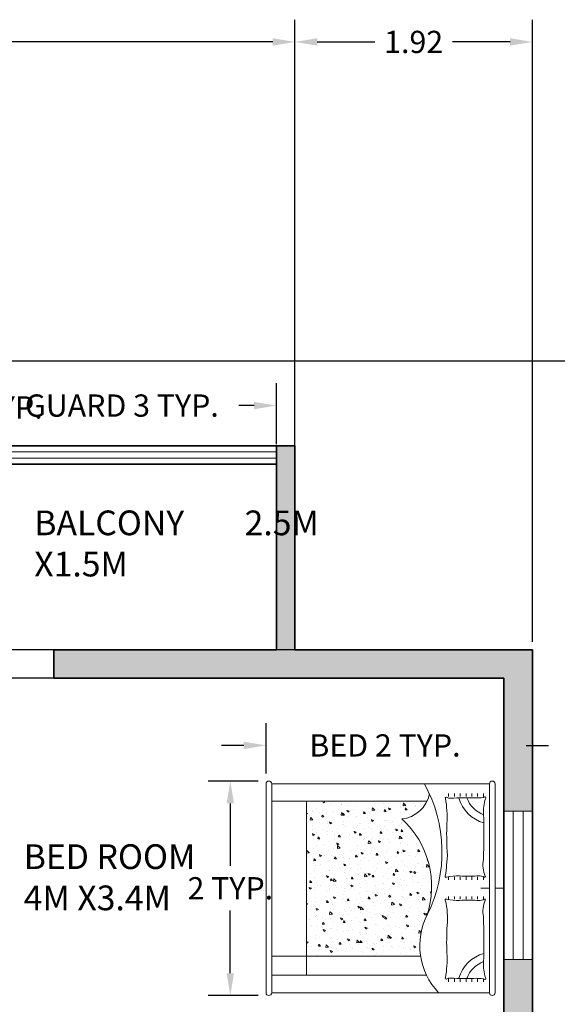
# Model space of a CAD drawing. Units: metres. Extents: x 2031 to 2061.8, y 1886.4 to 1909.8.
# Tile 10 of 10: x 2052.1 to 2056.4, y 1901.9 to 1909.8. Entities that reach past the tile are written whole.
import ezdxf

# ---------------------------------------------------------------- set-up
doc = ezdxf.new("R2010")
doc.units = ezdxf.units.M
for name, color, linetype, lineweight in [('A-ANNO-DIMS', 2, 'Continuous', 18), ('A-AREA-IDEN', 7, 'Continuous', 18), ('A-WALL-PATT', 252, 'Continuous', 13), ('furniture', 24, 'Continuous', 13), ('grills', 5, 'Continuous', 13), ('windows', 30, 'Continuous', 18)]:
    doc.layers.add(name, color=color, linetype=linetype, lineweight=lineweight)
doc.layers.add('outer walls', color=1, linetype='Continuous', lineweight=35, plot=False)
doc.styles.get("Standard").update_dxf_attribs({"font": 'arial.ttf'})
doc.dimstyles.get("Standard").update_dxf_attribs({"dimtxt": 0.18, "dimasz": 0.18, "dimexe": 0.18, "dimexo": 0.0625, "dimgap": 0.09, "dimtad": 0, "dimtih": 1, "dimtoh": 1, "dimdec": 4, "dimzin": 0, "dimdsep": 46, "dimtxsty": 'Standard', "dimcen": 0.09, "dimadec": 0, "dimazin": 0, "dimtfac": 1, "dimtdec": 4, "dimtofl": 0, "dimtmove": 0, "dimatfit": 3, "dimfxl": 1, "dimtolj": 1, "dimtzin": 0, "dimarcsym": 0})

# ---------------------------------------------------------------- blocks, each defined once
blk = doc.blocks.new('bed')
at = {"layer": 'furniture'}
h = blk.add_hatch(dxfattribs=at)
h.set_pattern_fill('AR-CONC', color=256, angle=-90.00000000000003, style=0)
h.set_pattern_definition([(320, (0, 2.380000000001032), (-0.6275213498259539, -7.172601826007534), [0.75, -8.25]), (265, (0, 2.380000000001032), (7.521921337000119, 1.387513336129997), [0.6, -6.599999999999999]), (10.45139999999999, (-0.0522933999999964, 1.782283200001032), (6.894395420609534, -5.785093817140218), [0.6374019000000001, -7.011421119999999]), (316.1842, (2, 2.380000000001032), (-1.655190143290184, -10.67241048625644), [1.125, -12.375]), (6.635599999999979, (1.862066929999997, 1.490632550001038), (9.741178709004412, -9.346627055487035), [0.956102879999999, -10.51712999999998]), (261.1842, (2, 2.380000000001032), (9.741186009253243, -9.346619451336275), [0.8999999999999989, -9.899999999999984]), (291, (1.5, 1.380000000001032), (-4.02618890665339, -5.969070521184614), [0.75, -8.25]), (236, (1.5, 1.380000000001032), (7.251500450468529, -2.433153319215819), [0.6, -6.599999999999999]), (341.4514, (1.164483939999996, 0.8825776700010266), (3.22530496709952, -8.402226285814901), [0.6374019000000001, -7.011421119999999]), (307.4999999999999, (0, 2.380000000001032), (3.328938538313114, -0.121598553172908), [0, -6.519999999999999, 0, -6.7, 0, -6.625]), (277.5, (0, 2.380000000001032), (3.944117118823601, -2.630695374421487), [0, -3.819999999999999, 0, -6.37, 0, -2.524999999999999]), (237.5, (0, 4.610000000001036), (-0.2255487173438, -5.33822436172409), [0, -2.5, 0, -7.799999999999999, 0, -10.35]), (227.5, (0, 5.610000000001036), (1.001049823323174, -5.831861693423862), [0, -3.25, 0, -5.179999999999999, 0, -7.349999999999999])])
h.paths.add_polyline_path([(30.01221964123038, -67.99999999999999), (30.01221964123036, -26.4972098666525, 0.2630430180581192), (23.90476957024844, -35.1500155485824, 0.2934236934375176), (-9.177957282599145, -26.46678060096597, -0.1566832162072435), (-23.39221964123496, -28.71851562074189), (-23.39221964123494, -67.99999999999999)])
for p, q in [((0, -3), (0, 0)), ((36.01221964123033, -3), (-36.01221964123033, -3)), ((-36.01221964123033, -5.000000000000028), (-36.01221964123027, -80)), ((36.01221964123033, -5.000000000000042), (-36.01221964123033, -5.000000000000028)), ((0, -8.000000000000043), (0, -5.000000000000042)), ((36.01221964123039, -79.99999999999999), (36.01221964123033, -5.000000000000042)), ((-31.23716250644156, -7.067621994530554), (-32.23716250644157, -7.067621994530554)), ((-31.23716250644156, -9.067621994530555), (-32.23716250644157, -9.067621994530555)), ((-3.810600647213163, -7.067621994530554), (-2.810600647213163, -7.067621994530554)), ((-3.810600647213163, -9.067621994530555), (-2.810600647213163, -9.067621994530555)), ((3.894900133777696, -7.067621994530526), (2.894900133777696, -7.067621994530526)), ((3.894900133777696, -9.067621994530526), (2.894900133777696, -9.067621994530526)), ((31.62837541028949, -7.067621994530526), (32.62837541028949, -7.067621994530526)), ((31.62837541028949, -9.067621994530526), (32.62837541028949, -9.067621994530526)), ((-31.23716250644156, -11.06762199453055), (-32.23716250644157, -11.06762199453055)), ((-31.23716250644156, -13.06762199453055), (-32.23716250644157, -13.06762199453055)), ((-3.810600647213163, -11.06762199453055), (-2.810600647213163, -11.06762199453055)), ((-3.810600647213163, -13.06762199453055), (-2.810600647213163, -13.06762199453055)), ((3.894900133777696, -11.06762199453052), (2.894900133777696, -11.06762199453052)), ((3.894900133777696, -13.06762199453052), (2.894900133777696, -13.06762199453052)), ((31.62837541028949, -11.06762199453052), (32.62837541028949, -11.06762199453052)), ((31.62837541028949, -13.06762199453052), (32.62837541028949, -13.06762199453052)), ((-31.23716250644156, -15.06762199453055), (-32.23716250644157, -15.06762199453055)), ((-3.810600647213163, -15.06762199453055), (-2.810600647213163, -15.06762199453055)), ((3.894900133777696, -15.06762199453052), (2.894900133777696, -15.06762199453052)), ((31.62837541028949, -15.06762199453052), (32.62837541028949, -15.06762199453052)), ((-31.23716250644156, -17.06762199453055), (-32.23716250644157, -17.06762199453055)), ((-31.23716250644156, -19.06762199453055), (-32.23716250644157, -19.06762199453055)), ((-3.810600647213163, -17.06762199453055), (-2.810600647213163, -17.06762199453055)), ((-3.810600647213163, -19.06762199453055), (-2.810600647213163, -19.06762199453055)), ((3.894900133777696, -17.06762199453052), (2.894900133777696, -17.06762199453052)), ((3.894900133777696, -19.06762199453052), (2.894900133777696, -19.06762199453052)), ((31.62837541028949, -17.06762199453052), (32.62837541028949, -17.06762199453052)), ((31.62837541028949, -19.06762199453052), (32.62837541028949, -19.06762199453052)), ((-36.01221964123027, -80), (36.01221964123039, -79.99999999999997)), ((-36.01221964123027, -82), (36.01221964123039, -82))]:
    blk.add_line(p, q, dxfattribs=at)
at = {"layer": 'furniture', "ltscale": 5}
blk.add_line((-30.0122196412303, -26.65900214866815), (-30.01221964123028, -80), dxfattribs=at)
at = {"layer": 'furniture', "ltscale": 7}
blk.add_line((30.01221964123039, -79.99999999999999), (30.01221964123036, -26.4972098666525), dxfattribs=at)
at = {"layer": 'furniture', "ltscale": 0.3}
for p, q in [((-23.39221964123493, -80.00000000000003), (-23.39221964123496, -28.71851562074188)), ((-30.01221964123028, -67.99999999999999), (30.01221964123039, -67.99999999999999))]:
    blk.add_line(p, q, dxfattribs=at)
at = {"layer": 'furniture'}
for centre, radius, start, end in [((-35.95310404783035, -4.000000000000014), 1.001745802777857, 93.38313670775338, 266.6168632922466), ((35.95310404783047, -4.000000000000014), 1.001745802777857, 273.3831367077534, 86.61686329224663), ((-31.09685452420217, -6.56812628935117), 0.3815901177143176, 35.89755946985184, 208.6271807330242), ((-44.4434251214767, -13.85312857714783), 14.82374463825802, 27.16285943351717, 28.62718073212637), ((-26.34909713879518, 6.677823774407073), 13.75788850886336, 251.1782289026713, 273.3982224065857), ((-8.031939823939297, 2.030581047412752), 9.294330538692307, 258.8960367609226, 294.7184225587751), ((-4.029449448298862, -6.668977911985379), 0.2818061021667602, 335.7259061638442, 114.3030308467571), ((3.223958981487498, -9.94006998173215), 7.675076275868892, 155.7259061638442, 159.0146401085631), ((4.113748934860268, -6.668977911985379), 0.2818061021635516, 65.69696915417202, 204.2740938370052), ((-3.139659494904833, -9.940069981732137), 7.675076275868892, 20.98535989143595, 24.27409383615427), ((8.116239310533615, 2.030581047735168), 9.294330539002221, 245.2815774418415, 281.1039632384965), ((26.43339662535652, 6.677823774423444), 13.75788850886336, 266.6017775934111, 288.8217710973251), ((31.18115401076358, -6.568126289351184), 0.3815901177179044, 331.3728192669758, 144.1024405301472), ((44.52772460803806, -13.85312857714784), 14.82374463825802, 151.3728192678729, 152.8371405664821), ((-46.75951437957865, -9.65138206848897), 15.71579241958107, 357.4803608088326, 9.395608387614068), ((-34.45294545533051, -3.506108501804959), 9.853247350176973, 289.8695209624031, 338.9842964810487), ((-34.45294545533051, -3.506108501804959), 12.47479548168961, 286.0319050224358, 344.1205283884622), ((-18.01528168092849, -163.5963416214672), 156.7209082093599, 87.00321809951629, 92.74968346925495), ((0.254091396095987, -8.800915214962217), 4.494229367051207, 159.014640107615, 186.2730421081171), ((-32.81622258778788, -12.43616332427339), 28.77528664700029, 354.3784002715227, 6.27304210895588), ((-0.1697919095242355, -8.800915214962217), 4.494229367051207, 353.7269578918828, 20.98535989238499), ((32.90052207435963, -12.43616332427341), 28.77528664700055, 173.7269578910441, 185.6215997284773), ((18.09958116748922, -163.5963416214399), 156.7209082093326, 87.2503165307418, 92.99678190048373), ((34.53724494190226, -3.506108501789682), 12.47479548168961, 195.8794716115377, 253.9680949775642), ((34.53724494190226, -3.506108501789682), 9.853247350176973, 201.0157035189505, 250.1304790375968), ((46.84381386614001, -9.651382068520647), 15.71579241958353, 170.6043916115409, 182.5196391911672), ((-28.61556435462791, 31.03444768063454), 42.31456350822244, 266.4835611990511, 266.6487421238194), ((54.88285648445511, -13.16191061182081), 85.98801403775587, 178.1208768196816, 183.3613129440673), ((-54.79855699787332, -13.1619106118885), 85.98801403775471, 356.6386870559327, 1.87912318031836), ((28.69986384117891, 31.03444768073385), 42.31456350831875, 273.3512578762066, 273.5164388009489), ((12.27920019974715, -16.10835590841725), 16.48064095036883, 177.0317121189266, 192.8677860199701), ((-12.19490071317551, -16.10835590841725), 16.48064095036894, 347.1322139800299, 2.968287881073314), ((-31.05019458355673, -19.91479358257859), 0.2912925215689113, 147.6219291273817, 311.93432899363), ((-33.19532486499685, -18.55460390606353), 2.248727139855352, 327.6219291288709, 339.224552802207), ((-34.12771521855714, -18.41167218428833), 3.177308659740759, 342.7808628527732, 3.755021134780372), ((-24.39731400277299, -58.0065508966982), 38.42172354635978, 93.51643880178425, 99.67664784205135), ((-24.51665474671893, -56.06449133928439), 36.47600066328987, 86.48356119821578, 93.51643880178425), ((-18.48842024981553, 70.49496359167773), 90.23180174042126, 267.5920770069633, 273.6328801943956), ((-10.30534078399284, -44.95285539311296), 25.51674577343078, 75.95197577712642, 95.54518109318596), ((-3.947726608991956, -19.99033763805275), 0.2654728058058112, 231.9004795059564, 52.89022406852256), ((4.032026095563765, -19.99033763805275), 0.2654728058058112, 127.1097759314774, 308.0995204940429), ((7.570216687580227, -34.67789736270967), 14.86666553287629, 87.39755039330738, 103.1191401867811), ((11.43897390287765, -34.80624327566366), 15.31635237680183, 84.69404282866213, 102.035481886755), ((18.57271973638731, 70.4949635916777), 90.23180174042125, 266.3671198056044, 272.4079229930367), ((24.6009542333012, -56.0644913392844), 36.47600066328987, 86.48356119821578, 93.51643880178425), ((24.48161348934542, -58.00655089669821), 38.42172354635978, 80.32335215794863, 86.48356119821578), ((31.13449407013883, -19.91479358255678), 0.2912925215689113, 228.06567100637, 32.37807087261824), ((34.21201470513921, -18.41167218428845), 3.177308659740705, 176.2449788652196, 197.2191371472267), ((33.27962435157895, -18.55460390604825), 2.248727139855352, 200.775447197793, 212.378070871129), ((-19.78970084288576, -5.469494448941333), 23.52647715105876, 226.4060518471351, 297.4441169484015), ((12.50744191168894, -69.71437404891591), 48.3828132966499, 60.93454900685955, 116.3226601669859), ((0.602167516954296, -56.56840710701565), 31.65057281321388, 42.58740832788977, 108.5033645785765), ((34.6132349005153, -36.22659364526982), 10.76244628919441, 101.1719081394, 174.2590453022261), ((-35.95310404783035, -81), 1.001745802777857, 93.38313670775338, 266.6168632922466), ((35.95310404783044, -81), 1.001745802777857, 273.3831367077534, 86.61686329224663)]:
    blk.add_arc(centre, radius, start, end, dxfattribs=at)
blk = doc.blocks.new('WIN-1200')
for p, q in [((0.2299999999995634, 1.200000000000045), (-4.547e-13, 1.199999999999818)), ((0.0750000000007276, -2.274e-13), (0.0749999999995907, 1.200000000000045)), ((0.1550000000006548, -2.274e-13), (0.154999999999518, 1.200000000000045)), ((0.2300000000007003, 0), (6.821e-13, -2.274e-13))]:
    blk.add_line(p, q)
blk = doc.blocks.new('BALCONY-GUARD-2500')
for p, q in [((4.547e-13, 0.0500000000010914), (2.5, 0.0500000000006367)), ((4.547e-13, 6.821e-13), (2.5, 4.547e-13))]:
    blk.add_line(p, q)
blk = doc.blocks.new('*D22')
at = {"layer": 'A-ANNO-DIMS', "color": 0, "lineweight": -2, "transparency": 16777216}
for p, q in [((2051.65388605158, 1906.406583869398), (2051.65388605158, 1906.899083869398)), ((2054.15388605158, 1906.406583869398), (2054.15388605158, 1906.899083869398)), ((2051.83388605158, 1906.719083869398), (2051.958210744622, 1906.719083869398)), ((2053.97388605158, 1906.719083869398), (2053.849561358537, 1906.719083869398))]:
    blk.add_line(p, q, dxfattribs=at)
at = {"layer": 'A-ANNO-DIMS', "color": 0, "transparency": 16777216}
for points in [[(2051.83388605158, 1906.749083869398), (2051.83388605158, 1906.689083869398), (2051.65388605158, 1906.719083869398)], [(2053.97388605158, 1906.749083869398), (2053.97388605158, 1906.689083869398), (2054.15388605158, 1906.719083869398)]]:
    blk.add_solid(points, dxfattribs=at)
at = {"layer": 'Defpoints', "color": 0, "transparency": 16777216}
for p in [(2054.15388605158, 1906.719083869398), (2051.65388605158, 1906.344083869398), (2054.15388605158, 1906.344083869398)]:
    blk.add_point(p, dxfattribs=at)
at = {"layer": 'A-ANNO-DIMS', "color": 0, "transparency": 16777216, "insert": (2052.90388605158, 1906.719083869398), "char_height": 0.18, "attachment_point": 5}
blk.add_mtext('\\A1;GUARD 3 TYP.', dxfattribs=at)
blk = doc.blocks.new('*D23')
at = {"layer": 'A-ANNO-DIMS', "color": 0, "lineweight": -2, "transparency": 16777216}
for p, q in [((2051.278886051582, 1906.524083869399), (2051.278886051582, 1906.704083869399)), ((2051.278886051582, 1906.704083869399), (2051.458886051582, 1906.704083869399)), ((2051.591386051581, 1906.344083869399), (2051.098886051582, 1906.344083869399)), ((2051.591386051581, 1906.294083869399), (2051.098886051582, 1906.294083869399)), ((2051.278886051582, 1906.114083869398), (2051.278886051582, 1905.934083869398))]:
    blk.add_line(p, q, dxfattribs=at)
at = {"layer": 'A-ANNO-DIMS', "color": 0, "transparency": 16777216}
for points in [[(2051.248886051581, 1906.524083869399), (2051.308886051582, 1906.524083869399), (2051.278886051582, 1906.344083869399)], [(2051.248886051581, 1906.114083869398), (2051.308886051582, 1906.114083869398), (2051.278886051582, 1906.294083869399)]]:
    blk.add_solid(points, dxfattribs=at)
at = {"layer": 'Defpoints', "color": 0, "transparency": 16777216}
for p in [(2051.278886051582, 1906.344083869399), (2051.653886051581, 1906.344083869399), (2051.653886051581, 1906.294083869399)]:
    blk.add_point(p, dxfattribs=at)
at = {"layer": 'A-ANNO-DIMS', "color": 0, "transparency": 16777216, "insert": (2051.917051126616, 1906.704083869398), "char_height": 0.18, "attachment_point": 5}
blk.add_mtext('\\A1;0 TYP.', dxfattribs=at)
blk = doc.blocks.new('*D36')
at = {"layer": 'A-ANNO-DIMS', "color": 0, "lineweight": -2, "transparency": 16777216}
for p, q in [((2054.069797345789, 1903.743710811128), (2054.069797345789, 1904.149824116997)), ((2055.993886051581, 1903.743710811128), (2055.993886051581, 1904.149824116997)), ((2053.889797345789, 1903.969824116997), (2053.709797345789, 1903.969824116997)), ((2056.173886051581, 1903.969824116997), (2056.353886051581, 1903.969824116997))]:
    blk.add_line(p, q, dxfattribs=at)
at = {"layer": 'A-ANNO-DIMS', "color": 0, "transparency": 16777216}
for points in [[(2053.889797345789, 1903.999824116997), (2053.889797345789, 1903.939824116997), (2054.069797345789, 1903.969824116997)], [(2056.173886051581, 1903.999824116997), (2056.173886051581, 1903.939824116997), (2055.993886051581, 1903.969824116997)]]:
    blk.add_solid(points, dxfattribs=at)
at = {"layer": 'Defpoints', "color": 0, "transparency": 16777216}
for p in [(2055.993886051581, 1903.969824116997), (2054.069797345789, 1903.681210811128), (2055.993886051581, 1903.681210811128)]:
    blk.add_point(p, dxfattribs=at)
at = {"layer": 'A-ANNO-DIMS', "color": 0, "transparency": 16777216, "insert": (2055.031841698685, 1903.969824116997), "char_height": 0.18, "attachment_point": 5}
blk.add_mtext('\\A1;BED 2 TYP.', dxfattribs=at)
blk = doc.blocks.new('*D37')
at = {"layer": 'A-ANNO-DIMS', "color": 0, "lineweight": -2, "transparency": 16777216}
for p, q in [((2054.00729734579, 1903.681210811129), (2053.601184039922, 1903.681210811129)), ((2053.781184039922, 1903.501210811129), (2053.781184039922, 1902.994513610191)), ((2053.781184039922, 1902.126956927671), (2053.781184039922, 1902.633654128609)), ((2054.00729734579, 1901.94695692767), (2053.601184039922, 1901.94695692767))]:
    blk.add_line(p, q, dxfattribs=at)
at = {"layer": 'A-ANNO-DIMS', "color": 0, "transparency": 16777216}
for points in [[(2053.751184039922, 1903.501210811129), (2053.811184039922, 1903.501210811129), (2053.781184039922, 1903.681210811129)], [(2053.751184039922, 1902.126956927671), (2053.811184039922, 1902.126956927671), (2053.781184039922, 1901.94695692767)]]:
    blk.add_solid(points, dxfattribs=at)
at = {"layer": 'Defpoints', "color": 0, "transparency": 16777216}
for p in [(2053.781184039922, 1903.681210811129), (2054.06979734579, 1903.681210811129), (2054.06979734579, 1901.94695692767)]:
    blk.add_point(p, dxfattribs=at)
at = {"layer": 'A-ANNO-DIMS', "color": 0, "transparency": 16777216, "insert": (2053.781184039922, 1902.814083869398), "char_height": 0.18, "attachment_point": 5}
blk.add_mtext('\\A1;2 TYP.', dxfattribs=at)
blk = doc.blocks.new('*D45')
at = {"layer": 'A-ANNO-DIMS', "color": 0, "lineweight": -2, "transparency": 16777216}
for p, q in [((2047.556386000001, 1907.081203000001), (2061.614374000002, 1907.081203000001)), ((2061.434374000002, 1906.901203000001), (2061.434374000002, 1897.862029637791)), ((2061.434374000002, 1888.459050000001), (2061.434374000002, 1897.498223362211)), ((2054.286386000001, 1888.279050000001), (2061.614374000002, 1888.279050000001))]:
    blk.add_line(p, q, dxfattribs=at)
at = {"layer": 'A-ANNO-DIMS', "color": 0, "transparency": 16777216}
for points in [[(2061.404374000002, 1906.901203000001), (2061.464374000002, 1906.901203000001), (2061.434374000002, 1907.081203000001)], [(2061.404374000002, 1888.459050000001), (2061.464374000002, 1888.459050000001), (2061.434374000002, 1888.279050000001)]]:
    blk.add_solid(points, dxfattribs=at)
at = {"layer": 'Defpoints', "color": 0, "transparency": 16777216}
for p in [(2047.493886000001, 1907.081203000001), (2061.434374000002, 1907.081203000001), (2054.223886000001, 1888.279050000001)]:
    blk.add_point(p, dxfattribs=at)
at = {"layer": 'A-ANNO-DIMS', "color": 0, "transparency": 16777216, "insert": (2061.434374000002, 1897.6801265), "char_height": 0.18, "attachment_point": 5}
blk.add_mtext('\\A1;18.802', dxfattribs=at)
blk = doc.blocks.new('*D49')
at = {"layer": 'A-ANNO-DIMS', "color": 0, "lineweight": -2, "transparency": 16777216}
for p, q in [((2047.343886, 1907.143703), (2047.343886, 1909.84065)), ((2054.303886, 1906.456584), (2054.303886, 1909.84065)), ((2047.523886, 1909.66065), (2050.499677268759, 1909.66065)), ((2054.123886000001, 1909.66065), (2051.148094731242, 1909.66065))]:
    blk.add_line(p, q, dxfattribs=at)
at = {"layer": 'A-ANNO-DIMS', "color": 0, "transparency": 16777216}
for points in [[(2047.523886, 1909.69065), (2047.523886, 1909.63065), (2047.343886, 1909.66065)], [(2054.123886000001, 1909.69065), (2054.123886000001, 1909.63065), (2054.303886, 1909.66065)]]:
    blk.add_solid(points, dxfattribs=at)
at = {"layer": 'Defpoints', "color": 0, "transparency": 16777216}
for p in [(2054.303886, 1909.66065), (2047.343886, 1907.081203), (2054.303886, 1906.394084)]:
    blk.add_point(p, dxfattribs=at)
at = {"layer": 'A-ANNO-DIMS', "color": 0, "transparency": 16777216, "insert": (2050.823886, 1909.66065), "char_height": 0.18, "attachment_point": 5}
blk.add_mtext('\\A1;6.96', dxfattribs=at)
blk = doc.blocks.new('*D50')
at = {"layer": 'A-ANNO-DIMS', "color": 0, "lineweight": -2, "transparency": 16777216}
for p, q in [((2054.303886, 1904.806584), (2054.303886, 1909.84065)), ((2056.223886000001, 1904.806584), (2056.223886000001, 1909.84065)), ((2054.483886, 1909.66065), (2054.949499915416, 1909.66065)), ((2056.043886000001, 1909.66065), (2055.578272084584, 1909.66065))]:
    blk.add_line(p, q, dxfattribs=at)
at = {"layer": 'A-ANNO-DIMS', "color": 0, "transparency": 16777216}
for points in [[(2054.483886, 1909.69065), (2054.483886, 1909.63065), (2054.303886, 1909.66065)], [(2056.043886000001, 1909.69065), (2056.043886000001, 1909.63065), (2056.223886000001, 1909.66065)]]:
    blk.add_solid(points, dxfattribs=at)
at = {"layer": 'Defpoints', "color": 0, "transparency": 16777216}
for p in [(2056.223886000001, 1909.66065), (2054.303886, 1904.744084), (2056.223886000001, 1904.744084)]:
    blk.add_point(p, dxfattribs=at)
at = {"layer": 'A-ANNO-DIMS', "color": 0, "transparency": 16777216, "insert": (2055.263886, 1909.66065), "char_height": 0.18, "attachment_point": 5}
blk.add_mtext('\\A1;1.92', dxfattribs=at)
blk = doc.blocks.new('*D60')
at = {"layer": 'A-ANNO-DIMS', "color": 0, "lineweight": -2, "transparency": 16777216}
for p, q in [((2031.744780000002, 1904.924084000001), (2031.744780000002, 1905.104084000001)), ((2056.161386000001, 1904.744084), (2031.564780000002, 1904.744084)), ((2055.931386000001, 1904.514084000001), (2031.564780000002, 1904.514084000001)), ((2031.744780000002, 1904.334084000001), (2031.744780000002, 1904.154084000001)), ((2031.744780000002, 1904.154084000001), (2031.564780000002, 1904.154084000001))]:
    blk.add_line(p, q, dxfattribs=at)
at = {"layer": 'A-ANNO-DIMS', "color": 0, "transparency": 16777216}
for points in [[(2031.714780000002, 1904.924084000001), (2031.774780000002, 1904.924084000001), (2031.744780000002, 1904.744084)], [(2031.714780000002, 1904.334084000001), (2031.774780000002, 1904.334084000001), (2031.744780000002, 1904.514084000001)]]:
    blk.add_solid(points, dxfattribs=at)
at = {"layer": 'Defpoints', "color": 0, "transparency": 16777216}
for p in [(2056.223886000001, 1904.744084), (2031.744780000002, 1904.514084000001), (2055.993886000001, 1904.514084000001)]:
    blk.add_point(p, dxfattribs=at)
at = {"layer": 'A-ANNO-DIMS', "color": 0, "transparency": 16777216, "insert": (2031.241001009552, 1904.154084), "char_height": 0.18, "attachment_point": 5}
blk.add_mtext('\\A1;0.23', dxfattribs=at)

msp = doc.modelspace()

# ---------------------------------------------------------------- hatches: boundary and pattern name
at = {"layer": 'A-WALL-PATT'}
h = msp.add_hatch(color=256, dxfattribs=at)
h.dxf.hatch_style = 1
h.paths.add_polyline_path([(2055.723886051581, 1899.601202985826), (2054.382747959846, 1899.601202985826), (2054.382747959846, 1900.884083869399), (2056.223886051581, 1900.884083869399), (2056.223886051581, 1902.238485983749), (2055.993886051581, 1902.238485983749), (2055.993886051581, 1901.1140838694), (2054.152747959847, 1901.1140838694), (2054.152747959847, 1899.684083882831), (2051.671801362485, 1899.684083882831), (2051.668720550386, 1900.463086761322), (2051.518721723415, 1900.462493543744), (2051.522127968044, 1899.601202985826), (2051.010160422872, 1899.601202985826), (2051.010160422872, 1899.371202985826), (2054.723886051581, 1899.371202985826), (2055.493886051581, 1899.371202985826), (2055.493886051581, 1895.571212564149), (2052.04003795628, 1895.571212564149), (2052.04003795628, 1895.334826264002), (2055.723886051581, 1895.334826264003)])
h.paths.add_polyline_path([(2056.223886051581, 1904.7440838694), (2054.30388605158, 1904.7440838694), (2054.30388605158, 1906.394083869399), (2054.15388605158, 1906.394083869399), (2054.15388605158, 1904.7440838694), (2052.35388605158, 1904.744083869399), (2052.35388605158, 1904.5140838694), (2055.993886051581, 1904.514083869399), (2055.993886051581, 1903.438485983748), (2056.223886051581, 1903.438485983749)])
h.paths.add_polyline_path([(2051.65388605158, 1906.394083869399), (2051.50388605158, 1906.394083869399), (2051.50388605158, 1904.7440838694), (2051.073484427694, 1904.7440838694), (2051.073484427694, 1904.5140838694), (2051.50388605158, 1904.5140838694), (2051.50388605158, 1903.2140838694), (2051.65388605158, 1903.2140838694), (2051.65388605158, 1904.514083869399), (2051.65388605158, 1904.744083869399)])
h.paths.add_polyline_path([(2050.573484427694, 1904.7440838694), (2049.259724738491, 1904.7440838694), (2049.259724738491, 1904.5140838694), (2049.85388605158, 1904.5140838694), (2049.85388605158, 1902.3640838694), (2051.657247644143, 1902.3640838694), (2051.656654421926, 1902.5140838694), (2051.54888605158, 1902.5140838694), (2050.00388605158, 1902.5140838694), (2050.00388605158, 1903.102134348594), (2050.00388605158, 1904.5140838694), (2050.573484427694, 1904.5140838694)])
h.paths.add_polyline_path([(2048.259724738491, 1904.7440838694), (2047.49388605158, 1904.7440838694), (2047.493886051581, 1907.081202972395), (2047.343886051582, 1907.081202972395), (2047.343886051581, 1901.835524324617), (2047.57388605158, 1901.835524324617), (2047.57388605158, 1902.134083869399), (2048.085735884881, 1902.134128710869), (2048.085735884882, 1902.284083869396), (2047.573886051581, 1902.2840838694), (2047.57388605158, 1904.5140838694), (2048.259724738491, 1904.5140838694)])
h.paths.add_polyline_path([(2047.57388605158, 1900.752643427613), (2047.34388605158, 1900.752643427612), (2047.34388605158, 1899.371202985826), (2047.57388605158, 1899.371202985826), (2047.57388605158, 1899.551202985826)])
h.paths.add_polyline_path([(2049.810160422872, 1899.601202985827), (2048.77388605158, 1899.601202985827), (2048.77388605158, 1899.371202985826), (2049.810160422872, 1899.371202985826)])

# ---------------------------------------------------------------- linework, layer by layer
at = {"layer": 'outer walls'}
for p, q in [((2051.50388605158, 1906.394083869399), (2054.30388605158, 1906.394083869399)), ((2054.15388605158, 1904.744083869399), (2054.15388605158, 1906.3940838694)), ((2054.30388605158, 1904.744083869399), (2054.30388605158, 1906.394083869399)), ((2051.65388605158, 1906.244083869399), (2054.15388605158, 1906.244083869399)), ((2052.35388605158, 1904.744083869399), (2054.15388605158, 1904.7440838694)), ((2052.35388605158, 1904.514083869399), (2052.35388605158, 1904.744083869399)), ((2054.30388605158, 1904.7440838694), (2056.223886051581, 1904.7440838694)), ((2056.223886051581, 1904.7440838694), (2056.223886051581, 1900.884083869399)), ((2052.35388605158, 1904.5140838694), (2055.993886051581, 1904.514083869399)), ((2055.993886051581, 1904.514083869399), (2055.993886051581, 1901.1140838694))]:
    msp.add_line(p, q, dxfattribs=at)

# ---------------------------------------------------------------- block references
at = {"layer": 'furniture', "xscale": -0.023464496412097, "yscale": 0.023464496412097, "zscale": 0.023464496412097, "rotation": 270}
msp.add_blockref('bed', (2055.993886051581, 1902.814083869399), dxfattribs=at)
at = {"layer": 'grills'}
msp.add_blockref('BALCONY-GUARD-2500', (2051.65388605158, 1906.294083869397), dxfattribs=at)
at = {"layer": 'windows'}
msp.add_blockref('WIN-1200', (2055.993886051581, 1902.238485983749), dxfattribs=at)

# ---------------------------------------------------------------- texts
at = {"layer": 'A-AREA-IDEN', "char_height": 0.2, "attachment_point": 7}
for s, insert in [('BALCONY        2.5M X1.5M', (2052.196132477277, 1905.33669712566)), ('   BED ROOM\\P   4M X3.4M', (2051.92694814376, 1902.636374541281))]:
    msp.add_mtext_dynamic_manual_height_columns(s, width=2.302330104705106, gutter_width=12.5, heights=[0], dxfattribs=dict(at, insert=insert))

# ---------------------------------------------------------------- dimensions: what is measured, and where the dimension line sits
at = {"layer": 'A-ANNO-DIMS'}
for base, p1, p2, picture, middle in [((2054.303886, 1909.66065), (2047.343886, 1907.081203), (2054.303886, 1906.394084), '*D49', (2050.823886, 1909.66065)), ((2056.223886000001, 1909.66065), (2054.303886, 1904.744084), (2056.223886000001, 1904.744084), '*D50', (2055.263886, 1909.66065))]:
    dim = msp.add_linear_dim(base=base, p1=p1, p2=p2, dimstyle='Standard', override={"dimdec": 2, "dimlfac": 1, "dimrnd": 0, "dimzin": 0, "dimdsep": 46, "dimlunit": 2}, dxfattribs=at)
    dim.commit()
    dim.dimension.update_dxf_attribs({"geometry": picture, "text_midpoint": middle})
for base, p1, p2, text, picture, middle in [((2054.15388605158, 1906.719083869398), (2051.65388605158, 1906.344083869398), (2054.15388605158, 1906.344083869398), 'GUARD <> TYP.', '*D22', (2052.90388605158, 1906.719083869398)), ((2055.993886051581, 1903.969824116997), (2054.069797345789, 1903.681210811128), (2055.993886051581, 1903.681210811128), 'BED <> TYP.', '*D36', (2055.031841698685, 1903.969824116997))]:
    dim = msp.add_linear_dim(base=base, p1=p1, p2=p2, text=text, dimstyle='Standard', override={"dimdec": 0, "dimlfac": 1, "dimrnd": 0, "dimzin": 0, "dimdsep": 46, "dimlunit": 2}, dxfattribs=at)
    dim.commit()
    dim.dimension.update_dxf_attribs({"geometry": picture, "text_midpoint": middle})
for base, p1, p2, override, picture, middle in [((2061.434374000002, 1907.081203000001), (2054.223886, 1888.27905), (2047.493886, 1907.081203), {"dimdec": 3, "dimlfac": 1, "dimrnd": 0, "dimzin": 0, "dimdsep": 46, "dimlunit": 2}, '*D45', (2061.434374000002, 1897.6801265)), ((2031.744780000002, 1904.514084000001), (2056.223886000001, 1904.744084), (2055.993886, 1904.514084), {"dimdec": 2, "dimlfac": 1, "dimrnd": 0, "dimzin": 0, "dimdsep": 46, "dimlunit": 2}, '*D60', (2031.241001009552, 1904.154084))]:
    dim = msp.add_linear_dim(base=base, p1=p1, p2=p2, angle=90, dimstyle='Standard', override=override, dxfattribs=at)
    dim.commit()
    dim.dimension.update_dxf_attribs({"geometry": picture, "text_midpoint": middle})
for base, p1, p2, picture, middle in [((2051.278886051582, 1906.344083869399), (2051.65388605158, 1906.294083869397), (2051.65388605158, 1906.344083869398), '*D23', (2051.917051126616, 1906.704083869398)), ((2053.781184039922, 1903.681210811129), (2054.069797345789, 1901.94695692767), (2054.069797345789, 1903.681210811128), '*D37', (2053.781184039922, 1902.814083869398))]:
    dim = msp.add_linear_dim(base=base, p1=p1, p2=p2, angle=90, text='<> TYP.', dimstyle='Standard', override={"dimdec": 0, "dimlfac": 1, "dimrnd": 0, "dimzin": 0, "dimdsep": 46, "dimlunit": 2}, dxfattribs=at)
    dim.commit()
    dim.dimension.update_dxf_attribs({"geometry": picture, "text_midpoint": middle})

doc.saveas('drawing.dxf')
